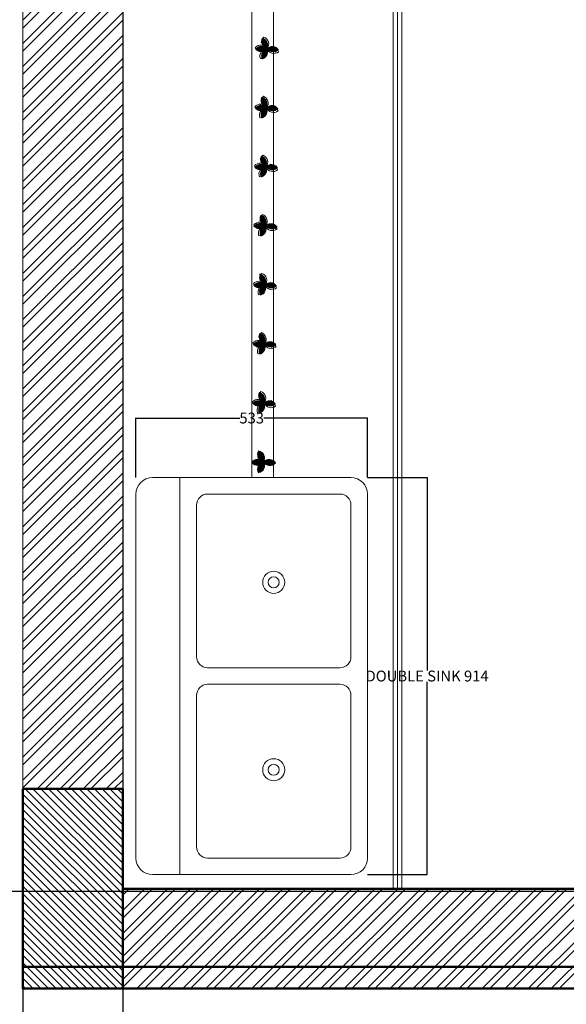
# Model space of a CAD drawing. Units: millimetres. Extents: x 1944 to 29915, y -10550 to 5909.
# Tile 4 of 24: x 6709 to 7967, y -5 to 2263. Entities that reach past the tile are written whole.
import ezdxf
from ezdxf import colors
from ezdxf.entities.mleader import LeaderData, LeaderLine
from ezdxf.math import Vec2, Vec3

# ---------------------------------------------------------------- set-up
doc = ezdxf.new("R2010")
doc.units = ezdxf.units.MM
doc.header["$MEASUREMENT"] = 0
for name, color, linetype, lineweight in [('A-ANNO-DIMS', 2, 'Continuous', 18), ('A-ANNO-TEXT', 7, 'Continuous', 25), ('A-FLOR-FIXT', 9, 'Continuous', 18), ('A-FLOR-PATT', 252, 'Continuous', 13), ('A-WALL', 7, 'Continuous', 50), ('A-WALL-PATT', 8, 'Continuous', 18)]:
    doc.layers.add(name, color=color, linetype=linetype, lineweight=lineweight)
doc.styles.get("Standard").update_dxf_attribs({"font": 'arial.ttf'})
doc.dimstyles.get("Standard").update_dxf_attribs({"dimtxt": 25, "dimasz": 0.18, "dimexe": 0.18, "dimexo": 0.0625, "dimgap": 0.09, "dimtad": 0, "dimtih": 1, "dimtoh": 1, "dimdec": 0, "dimzin": 0, "dimdsep": 46, "dimtxsty": 'Standard', "dimcen": 0.09, "dimadec": 0, "dimazin": 0, "dimtfac": 1, "dimtdec": 0, "dimtofl": 0, "dimtmove": 0, "dimatfit": 3, "dimfxl": 1, "dimtolj": 1, "dimtzin": 0, "dimarcsym": 0})

# ---------------------------------------------------------------- blocks, each defined once
blk = doc.blocks.new('Sink-double - 36 in top')
for p, q in [((-18, -4), (18, -4)), ((-0.75, -18.5), (-0.75, -6.5)), ((0.75, -6.5), (0.75, -18.5))]:
    blk.add_line(p, q)
for points in [[(-16.5, 0), (16.5, 0)], [(-18, -19.5), (-18, -1.5)], [(18, -1.5), (18, -19.5)], [(-15.5, -5.5), (-1.75, -5.5)], [(1.75, -5.5), (15.5, -5.5)], [(-16.5, -18.5), (-16.5, -6.5)], [(16.5, -6.5), (16.5, -18.5)], [(-1.75, -19.5), (-15.5, -19.5)], [(15.5, -19.5), (1.75, -19.5)], [(16.5, -21), (-16.5, -21)]]:
    blk.add_lwpolyline(points)
for centre, radius in [((-8.5, -12.5), 1), ((8.5, -12.5), 1), ((-8.5, -12.5), 0.5), ((8.5, -12.5), 0.5)]:
    blk.add_circle(centre, radius)
for centre, radius, start, end in [((-16.5, -1.5), 1.5, 90, 180), ((16.5, -1.5), 1.5, 0, 90), ((-15.5, -6.5), 1, 90, 180), ((-1.75, -6.5), 1, 0, 90), ((1.75, -6.5), 1, 90, 180), ((15.5, -6.5), 1, 0, 90), ((-15.5, -18.5), 1, 180, 270), ((-1.75, -18.5), 1, 270, 0), ((1.75, -18.5), 1, 180, 270), ((15.5, -18.5), 1, 270, 0), ((-16.5, -19.5), 1.5, 180, 270), ((16.5, -19.5), 1.5, 270, 0)]:
    blk.add_arc(centre, radius, start, end)
blk = doc.blocks.new('ORNAMENT-TILE')
for points in [[(27, 25, 0.520567), (15.6, 50, 0.520567)], [(27.4, 25, -0.520567), (0, 23.1, -0.520567)], [(27, 25, -0.520567), (15.6, 0, -0.520567)], [(27, 25, 0.520567), (54.3, 22.2, 0.520567)]]:
    blk.add_lwpolyline(points, format="xyb", close=True)
blk = doc.blocks.new('*D42')
at = {"layer": 'A-ANNO-DIMS', "color": 0, "lineweight": -2, "transparency": 16777216}
for p, q in [((7509.6, 1208), (7646.9, 1208)), ((7646.7, 1207.8), (7646.7, 763.8)), ((7646.7, 293.7), (7646.7, 737.7)), ((7509.6, 293.6), (7646.9, 293.6))]:
    blk.add_line(p, q, dxfattribs=at)
at = {"layer": 'A-ANNO-DIMS', "color": 0, "transparency": 16777216}
for points in [[(7646.7, 1207.8), (7646.8, 1207.8), (7646.7, 1208)], [(7646.7, 293.7), (7646.8, 293.7), (7646.7, 293.6)]]:
    blk.add_solid(points, dxfattribs=at)
at = {"layer": 'Defpoints', "color": 0, "transparency": 16777216}
for p in [(7509.6, 1208), (7646.7, 1208), (7509.6, 293.6)]:
    blk.add_point(p, dxfattribs=at)
at = {"layer": 'A-ANNO-DIMS', "color": 0, "transparency": 16777216, "insert": (7646.7, 750.8), "char_height": 25, "attachment_point": 5}
blk.add_mtext('\\A1;DOUBLE SINK 914', dxfattribs=at)
blk = doc.blocks.new('*D43')
at = {"layer": 'A-ANNO-DIMS', "color": 0, "lineweight": -2, "transparency": 16777216}
for p, q in [((6976.2, 1208), (6976.2, 1345.3)), ((6976.3, 1345.1), (7215.2, 1345.1)), ((7509.4, 1345.1), (7270.6, 1345.1)), ((7509.6, 1208), (7509.6, 1345.3))]:
    blk.add_line(p, q, dxfattribs=at)
at = {"layer": 'A-ANNO-DIMS', "color": 0, "transparency": 16777216}
for points in [[(6976.3, 1345.2), (6976.3, 1345.1), (6976.2, 1345.1)], [(7509.4, 1345.2), (7509.4, 1345.1), (7509.6, 1345.1)]]:
    blk.add_solid(points, dxfattribs=at)
at = {"layer": 'Defpoints', "color": 0, "transparency": 16777216}
for p in [(6976.2, 1345.1), (6976.2, 1208), (7509.6, 1208)]:
    blk.add_point(p, dxfattribs=at)
at = {"layer": 'A-ANNO-DIMS', "color": 0, "transparency": 16777216, "insert": (7242.9, 1345.1), "char_height": 25, "attachment_point": 5}
blk.add_mtext('\\A1;533', dxfattribs=at)
blk = doc.blocks.new('*D49')
at = {"layer": 'A-ANNO-DIMS', "color": 0, "lineweight": -2, "transparency": 16777216}
for p, q in [((8335.5, 4760.8), (8335.5, -697.2)), ((6945.9, 4530.8), (6945.9, -697.2)), ((6946.1, -697), (7589.8, -697)), ((8335.3, -697), (7691.6, -697))]:
    blk.add_line(p, q, dxfattribs=at)
at = {"layer": 'A-ANNO-DIMS', "color": 0, "transparency": 16777216}
for points in [[(6946.1, -697), (6946.1, -697.1), (6945.9, -697)], [(8335.3, -697), (8335.3, -697.1), (8335.5, -697)]]:
    blk.add_solid(points, dxfattribs=at)
at = {"layer": 'Defpoints', "color": 0, "transparency": 16777216}
for p in [(8335.5, 4760.8), (6945.9, 4530.8), (8335.5, -697)]:
    blk.add_point(p, dxfattribs=at)
at = {"layer": 'A-ANNO-DIMS', "color": 0, "transparency": 16777216, "insert": (7640.7, -697), "char_height": 25, "attachment_point": 5}
blk.add_mtext('\\A1;1389.5', dxfattribs=at)
blk = doc.blocks.new('*D52')
at = {"layer": 'A-ANNO-DIMS', "color": 0, "lineweight": -2, "transparency": 16777216}
for p, q in [((6715.9, 490.8), (6715.9, -697.2)), ((6945.9, 490.8), (6945.9, -697.2)), ((6716.1, -697), (6803.1, -697)), ((6945.8, -697), (6858.8, -697))]:
    blk.add_line(p, q, dxfattribs=at)
at = {"layer": 'A-ANNO-DIMS', "color": 0, "transparency": 16777216}
for points in [[(6716.1, -697), (6716.1, -697.1), (6715.9, -697)], [(6945.8, -697), (6945.8, -697.1), (6945.9, -697)]]:
    blk.add_solid(points, dxfattribs=at)
at = {"layer": 'Defpoints', "color": 0, "transparency": 16777216}
for p in [(6715.9, 490.8), (6945.9, 490.8), (6945.9, -697)]:
    blk.add_point(p, dxfattribs=at)
at = {"layer": 'A-ANNO-DIMS', "color": 0, "transparency": 16777216, "insert": (6830.9, -697), "char_height": 25, "attachment_point": 5}
blk.add_mtext('\\A1;230', dxfattribs=at)
blk = doc.blocks.new('*D53')
at = {"layer": 'A-ANNO-DIMS', "color": 0, "lineweight": -2, "transparency": 16777216}
for p, q in [((6945.94205, 490.774608), (6945.94205, -697.212556)), ((9895.94205, 490.774608), (9895.94205, -697.212556)), ((6946.12205, -697.032556), (8383.35205, -697.032556)), ((9895.76205, -697.032556), (8458.53205, -697.032556))]:
    blk.add_line(p, q, dxfattribs=at)
at = {"layer": 'A-ANNO-DIMS', "color": 0, "transparency": 16777216}
for points in [[(6946.12205, -697.002556), (6946.12205, -697.062556), (6945.94205, -697.032556)], [(9895.76205, -697.002556), (9895.76205, -697.062556), (9895.94205, -697.032556)]]:
    blk.add_solid(points, dxfattribs=at)
at = {"layer": 'Defpoints', "color": 0, "transparency": 16777216}
for p in [(6945.94205, 490.837108), (9895.94205, 490.837108), (9895.94205, -697.032556)]:
    blk.add_point(p, dxfattribs=at)
at = {"layer": 'A-ANNO-DIMS', "color": 0, "transparency": 16777216, "insert": (8420.94205, -697.032556), "char_height": 25, "attachment_point": 5}
blk.add_mtext('\\A1;2950', dxfattribs=at)
blk = doc.blocks.new('*D57')
at = {"layer": 'A-ANNO-DIMS', "color": 0, "lineweight": -2, "transparency": 16777216}
for p, q in [((8995.2, 4760.8), (5803.8, 4760.8)), ((5804, 4760.7), (5804, 2520.7)), ((5804, 255), (5804, 2495)), ((8999.6, 254.8), (5803.8, 254.8))]:
    blk.add_line(p, q, dxfattribs=at)
at = {"layer": 'A-ANNO-DIMS', "color": 0, "transparency": 16777216}
for points in [[(5804, 4760.7), (5804, 4760.7), (5804, 4760.8)], [(5804, 255), (5804, 255), (5804, 254.8)]]:
    blk.add_solid(points, dxfattribs=at)
at = {"layer": 'Defpoints', "color": 0, "transparency": 16777216}
for p in [(8995.2, 4760.8), (5804, 254.8), (8999.6, 254.8)]:
    blk.add_point(p, dxfattribs=at)
at = {"layer": 'A-ANNO-DIMS', "color": 0, "transparency": 16777216, "insert": (5804, 2507.8), "char_height": 25, "attachment_point": 5}
blk.add_mtext('\\A1;4506', dxfattribs=at)

msp = doc.modelspace()

# ---------------------------------------------------------------- hatches: boundary and pattern name
at = {"layer": 'A-FLOR-PATT'}
h = msp.add_hatch(dxfattribs=at)
h.set_pattern_fill('ANSI32', color=256, scale=100)
h.paths.add_polyline_path([(7278.336, 2195.885, -0.00568537), (7278.146, 2196.216, 0.21614784), (7266.8, 2188.29, 0.21566285)], flags=16)
h.paths.add_polyline_path([(7305.459, 2193.46, -0.51336232), (7278.336, 2195.885, -0.51336232), (7266.78, 2171.228, -0.27363046), (7266.8, 2188.29, -0.26802551), (7251.152, 2194.293, -0.30570263), (7268.133, 2202.214, -0.18072738), (7278.345, 2196.442, -0.51487633)])
h.paths.add_polyline_path([(7278.336, 2195.885, -0.21566285), (7266.8, 2188.29, 0.27363046), (7266.78, 2171.228, 0.51336232)], flags=16)
h = msp.add_hatch(dxfattribs=at)
h.set_pattern_fill('ANSI32', color=256, scale=100)
h.paths.add_polyline_path([(7278.146, 2196.216, -0.17977754), (7268.133, 2202.214, 0.30570263), (7251.152, 2194.293, 0.26802551), (7266.8, 2188.29, -0.21614784)])
h.paths.add_polyline_path([(7278.336, 2195.885, -0.00568537), (7278.146, 2196.216, 0.21614784), (7266.8, 2188.29, 0.21566285)], flags=16)
h.paths.add_polyline_path([(7278.336, 2195.885, -0.21566285), (7266.8, 2188.29, 0.27363046), (7266.78, 2171.228, 0.51336232)], flags=16)
h = msp.add_hatch(color=256, dxfattribs=at)
h.dxf.hatch_style = 1
h.paths.add_polyline_path([(7268.133, 2202.214, 0.30570263), (7251.152, 2194.293, 0.26802551), (7266.8, 2188.29, -0.21614784), (7278.146, 2196.216, -0.17977754)])
h = msp.add_hatch(dxfattribs=at)
h.set_pattern_fill('ANSI32', color=256, scale=100)
h.paths.add_polyline_path([(7266.78, 2221.204, 0.31162563), (7268.133, 2202.214, -0.17976414), (7278.304, 2196.49, 0.51458497)])
h = msp.add_hatch(color=256, dxfattribs=at)
h.dxf.hatch_style = 1
h.paths.add_polyline_path([(7266.78, 2221.204, 0.31162563), (7268.133, 2202.214, -0.17976414), (7278.304, 2196.49, 0.51458497)])
h = msp.add_hatch(color=256, dxfattribs=at)
h.dxf.hatch_style = 1
h.paths.add_polyline_path([(7268.133, 2202.214, -0.17976414), (7278.304, 2196.49, 0.51458497), (7266.78, 2221.204, 0.31162563)])
h = msp.add_hatch(color=256, dxfattribs=at)
h.dxf.hatch_style = 1
h.paths.add_polyline_path([(7268.133, 2202.214, 0.17977754), (7278.146, 2196.216, 0.00471819), (7278.304, 2196.49, 0.17976414)])
h = msp.add_hatch(color=256, dxfattribs=at)
h.dxf.hatch_style = 1
h.paths.add_polyline_path([(7278.345, 2196.442, -0.00448785), (7278.536, 2196.21, -0.00568537), (7278.336, 2195.885, 0.51336232), (7305.459, 2193.46, 0.51487633)])
h = msp.add_hatch(color=256, dxfattribs=at)
h.dxf.hatch_style = 1
h.paths.add_polyline_path([(7266.8, 2188.29, 0.27363046), (7266.78, 2171.228, 0.51336232), (7278.336, 2195.885, -0.21566285)])
h = msp.add_hatch(color=256, dxfattribs=at)
h.dxf.hatch_style = 1
h.paths.add_polyline_path([(7278.336, 2195.885, -0.00568537), (7278.146, 2196.216, 0.21614784), (7266.8, 2188.29, 0.21566285)])
h = msp.add_hatch(dxfattribs=at)
h.set_pattern_fill('ANSI32', color=256, scale=100)
h.paths.add_polyline_path([(7277.206, 2059.88, -0.00568537), (7277.016, 2060.21, 0.21614784), (7265.67, 2052.285, 0.21566285)], flags=16)
h.paths.add_polyline_path([(7304.329, 2057.455, -0.51336232), (7277.206, 2059.88, -0.51336232), (7265.651, 2035.222, -0.27363046), (7265.67, 2052.285, -0.26802551), (7250.022, 2058.288, -0.30570263), (7267.004, 2066.209, -0.18072738), (7277.215, 2060.436, -0.51487633)])
h.paths.add_polyline_path([(7277.206, 2059.88, -0.21566285), (7265.67, 2052.285, 0.27363046), (7265.651, 2035.222, 0.51336232)], flags=16)
h = msp.add_hatch(dxfattribs=at)
h.set_pattern_fill('ANSI32', color=256, scale=100)
h.paths.add_polyline_path([(7277.016, 2060.21, -0.17977754), (7267.004, 2066.209, 0.30570263), (7250.022, 2058.288, 0.26802551), (7265.67, 2052.285, -0.21614784)])
h.paths.add_polyline_path([(7277.206, 2059.88, -0.00568537), (7277.016, 2060.21, 0.21614784), (7265.67, 2052.285, 0.21566285)], flags=16)
h.paths.add_polyline_path([(7277.206, 2059.88, -0.21566285), (7265.67, 2052.285, 0.27363046), (7265.651, 2035.222, 0.51336232)], flags=16)
h = msp.add_hatch(color=256, dxfattribs=at)
h.dxf.hatch_style = 1
h.paths.add_polyline_path([(7267.004, 2066.209, 0.30570263), (7250.022, 2058.288, 0.26802551), (7265.67, 2052.285, -0.21614784), (7277.016, 2060.21, -0.17977754)])
h = msp.add_hatch(dxfattribs=at)
h.set_pattern_fill('ANSI32', color=256, scale=100)
h.paths.add_polyline_path([(7265.651, 2085.198, 0.31162563), (7267.004, 2066.209, -0.17976414), (7277.175, 2060.484, 0.51458497)])
h = msp.add_hatch(color=256, dxfattribs=at)
h.dxf.hatch_style = 1
h.paths.add_polyline_path([(7265.651, 2085.198, 0.31162563), (7267.004, 2066.209, -0.17976414), (7277.175, 2060.484, 0.51458497)])
h = msp.add_hatch(color=256, dxfattribs=at)
h.dxf.hatch_style = 1
h.paths.add_polyline_path([(7265.651, 2085.198, 0.31162563), (7267.004, 2066.209, -0.17976414), (7277.175, 2060.484, 0.51458497)])
h = msp.add_hatch(color=256, dxfattribs=at)
h.dxf.hatch_style = 1
h.paths.add_polyline_path([(7267.004, 2066.209, 0.17977754), (7277.016, 2060.21, 0.00471819), (7277.175, 2060.484, 0.17976414)])
h = msp.add_hatch(color=256, dxfattribs=at)
h.dxf.hatch_style = 1
h.paths.add_polyline_path([(7277.215, 2060.436, -0.00448785), (7277.406, 2060.204, -0.00568537), (7277.206, 2059.88, 0.51336232), (7304.329, 2057.455, 0.51487633)])
h = msp.add_hatch(color=256, dxfattribs=at)
h.dxf.hatch_style = 1
h.paths.add_polyline_path([(7265.67, 2052.285, 0.27363046), (7265.651, 2035.222, 0.51336232), (7277.206, 2059.88, -0.21566285)])
h = msp.add_hatch(color=256, dxfattribs=at)
h.dxf.hatch_style = 1
h.paths.add_polyline_path([(7277.206, 2059.88, -0.00568537), (7277.016, 2060.21, 0.21614784), (7265.67, 2052.285, 0.21566285)])
h = msp.add_hatch(dxfattribs=at)
h.set_pattern_fill('ANSI32', color=256, scale=100)
h.paths.add_polyline_path([(7276.077, 1923.875, -0.00568537), (7275.887, 1924.205, 0.21614784), (7264.54, 1916.279, 0.21566285)], flags=16)
h.paths.add_polyline_path([(7303.199, 1921.449, -0.51336232), (7276.077, 1923.875, -0.51336232), (7264.521, 1899.217, -0.27363046), (7264.54, 1916.279, -0.26802551), (7248.892, 1922.282, -0.30570263), (7265.874, 1930.203, -0.18072738), (7276.085, 1924.431, -0.51487633)])
h.paths.add_polyline_path([(7276.077, 1923.875, -0.21566285), (7264.54, 1916.279, 0.27363046), (7264.521, 1899.217, 0.51336232)], flags=16)
h = msp.add_hatch(dxfattribs=at)
h.set_pattern_fill('ANSI32', color=256, scale=100)
h.paths.add_polyline_path([(7275.887, 1924.205, -0.17977754), (7265.874, 1930.203, 0.30570263), (7248.892, 1922.282, 0.26802551), (7264.54, 1916.279, -0.21614784)])
h.paths.add_polyline_path([(7276.077, 1923.875, -0.00568537), (7275.887, 1924.205, 0.21614784), (7264.54, 1916.279, 0.21566285)], flags=16)
h.paths.add_polyline_path([(7276.077, 1923.875, -0.21566285), (7264.54, 1916.279, 0.27363046), (7264.521, 1899.217, 0.51336232)], flags=16)
h = msp.add_hatch(color=256, dxfattribs=at)
h.dxf.hatch_style = 1
h.paths.add_polyline_path([(7265.874, 1930.203, 0.30570263), (7248.892, 1922.282, 0.26802551), (7264.54, 1916.279, -0.21614784), (7275.887, 1924.205, -0.17977754)])
h = msp.add_hatch(dxfattribs=at)
h.set_pattern_fill('ANSI32', color=256, scale=100)
h.paths.add_polyline_path([(7264.521, 1949.193, 0.31162563), (7265.874, 1930.203, -0.17976414), (7276.045, 1924.479, 0.51458497)])
h = msp.add_hatch(color=256, dxfattribs=at)
h.dxf.hatch_style = 1
h.paths.add_polyline_path([(7264.521, 1949.193, 0.31162563), (7265.874, 1930.203, -0.17976414), (7276.045, 1924.479, 0.51458497)])
h = msp.add_hatch(color=256, dxfattribs=at)
h.dxf.hatch_style = 1
h.paths.add_polyline_path([(7264.521, 1949.193, 0.31162563), (7265.874, 1930.203, -0.17976414), (7276.045, 1924.479, 0.51458497)])
h = msp.add_hatch(color=256, dxfattribs=at)
h.dxf.hatch_style = 1
h.paths.add_polyline_path([(7265.874, 1930.203, 0.17977754), (7275.887, 1924.205, 0.00471819), (7276.045, 1924.479, 0.17976414)])
h = msp.add_hatch(color=256, dxfattribs=at)
h.dxf.hatch_style = 1
h.paths.add_polyline_path([(7276.085, 1924.431, -0.00448785), (7276.276, 1924.199, -0.00568537), (7276.077, 1923.875, 0.51336232), (7303.199, 1921.449, 0.51487633)])
h = msp.add_hatch(color=256, dxfattribs=at)
h.dxf.hatch_style = 1
h.paths.add_polyline_path([(7264.54, 1916.279, 0.27363046), (7264.521, 1899.217, 0.51336232), (7276.077, 1923.875, -0.21566285)])
h = msp.add_hatch(color=256, dxfattribs=at)
h.dxf.hatch_style = 1
h.paths.add_polyline_path([(7276.077, 1923.875, -0.00568537), (7275.887, 1924.205, 0.21614784), (7264.54, 1916.279, 0.21566285)])
h = msp.add_hatch(dxfattribs=at)
h.set_pattern_fill('ANSI32', color=256, scale=100)
h.paths.add_polyline_path([(7274.947, 1787.869, -0.00568537), (7274.757, 1788.2, 0.21614784), (7263.41, 1780.274, 0.21566285)], flags=16)
h.paths.add_polyline_path([(7302.069, 1785.444, -0.51336232), (7274.947, 1787.869, -0.51336232), (7263.391, 1763.212, -0.27363046), (7263.41, 1780.274, -0.26802551), (7247.762, 1786.277, -0.30570263), (7264.744, 1794.198, -0.18072738), (7274.955, 1788.426, -0.51487633)])
h.paths.add_polyline_path([(7274.947, 1787.869, -0.21566285), (7263.41, 1780.274, 0.27363046), (7263.391, 1763.212, 0.51336232)], flags=16)
h = msp.add_hatch(dxfattribs=at)
h.set_pattern_fill('ANSI32', color=256, scale=100)
h.paths.add_polyline_path([(7274.757, 1788.2, -0.17977754), (7264.744, 1794.198, 0.30570263), (7247.762, 1786.277, 0.26802551), (7263.41, 1780.274, -0.21614784)])
h.paths.add_polyline_path([(7274.947, 1787.869, -0.00568537), (7274.757, 1788.2, 0.21614784), (7263.41, 1780.274, 0.21566285)], flags=16)
h.paths.add_polyline_path([(7274.947, 1787.869, -0.21566285), (7263.41, 1780.274, 0.27363046), (7263.391, 1763.212, 0.51336232)], flags=16)
h = msp.add_hatch(color=256, dxfattribs=at)
h.dxf.hatch_style = 1
h.paths.add_polyline_path([(7264.744, 1794.198, 0.30570263), (7247.762, 1786.277, 0.26802551), (7263.41, 1780.274, -0.21614784), (7274.757, 1788.2, -0.17977754)])
h = msp.add_hatch(dxfattribs=at)
h.set_pattern_fill('ANSI32', color=256, scale=100)
h.paths.add_polyline_path([(7263.391, 1813.187, 0.31162563), (7264.744, 1794.198, -0.17976414), (7274.915, 1788.473, 0.51458497)])
h = msp.add_hatch(color=256, dxfattribs=at)
h.dxf.hatch_style = 1
h.paths.add_polyline_path([(7263.391, 1813.187, 0.31162563), (7264.744, 1794.198, -0.17976414), (7274.915, 1788.473, 0.51458497)])
h = msp.add_hatch(color=256, dxfattribs=at)
h.dxf.hatch_style = 1
h.paths.add_polyline_path([(7274.915, 1788.473, 0.51458497), (7263.391, 1813.187, 0.31162563), (7264.744, 1794.198, -0.17976414)])
h = msp.add_hatch(color=256, dxfattribs=at)
h.dxf.hatch_style = 1
h.paths.add_polyline_path([(7264.744, 1794.198, 0.17977754), (7274.757, 1788.2, 0.00471819), (7274.915, 1788.473, 0.17976414)])
h = msp.add_hatch(color=256, dxfattribs=at)
h.dxf.hatch_style = 1
h.paths.add_polyline_path([(7274.955, 1788.426, -0.00448785), (7275.147, 1788.194, -0.00568537), (7274.947, 1787.869, 0.51336232), (7302.069, 1785.444, 0.51487633)])
h = msp.add_hatch(color=256, dxfattribs=at)
h.dxf.hatch_style = 1
h.paths.add_polyline_path([(7263.41, 1780.274, 0.27363046), (7263.391, 1763.212, 0.51336232), (7274.947, 1787.869, -0.21566285)])
h = msp.add_hatch(color=256, dxfattribs=at)
h.dxf.hatch_style = 1
h.paths.add_polyline_path([(7274.947, 1787.869, -0.00568537), (7274.757, 1788.2, 0.21614784), (7263.41, 1780.274, 0.21566285)])
h = msp.add_hatch(dxfattribs=at)
h.set_pattern_fill('ANSI32', color=256, scale=100)
h.paths.add_polyline_path([(7273.817, 1651.864, -0.00568537), (7273.627, 1652.194, 0.21614784), (7262.281, 1644.268, 0.21566285)], flags=16)
h.paths.add_polyline_path([(7300.94, 1649.438, -0.51336232), (7273.817, 1651.864, -0.51336232), (7262.261, 1627.206, -0.27363046), (7262.281, 1644.268, -0.26802551), (7246.633, 1650.272, -0.30570263), (7263.614, 1658.193, -0.18072738), (7273.825, 1652.42, -0.51487633)])
h.paths.add_polyline_path([(7273.817, 1651.864, -0.21566285), (7262.281, 1644.268, 0.27363046), (7262.261, 1627.206, 0.51336232)], flags=16)
h = msp.add_hatch(dxfattribs=at)
h.set_pattern_fill('ANSI32', color=256, scale=100)
h.paths.add_polyline_path([(7273.627, 1652.194, -0.17977754), (7263.614, 1658.193, 0.30570263), (7246.633, 1650.272, 0.26802551), (7262.281, 1644.268, -0.21614784)])
h.paths.add_polyline_path([(7273.817, 1651.864, -0.00568537), (7273.627, 1652.194, 0.21614784), (7262.281, 1644.268, 0.21566285)], flags=16)
h.paths.add_polyline_path([(7273.817, 1651.864, -0.21566285), (7262.281, 1644.268, 0.27363046), (7262.261, 1627.206, 0.51336232)], flags=16)
h = msp.add_hatch(color=256, dxfattribs=at)
h.dxf.hatch_style = 1
h.paths.add_polyline_path([(7263.614, 1658.193, 0.30570263), (7246.633, 1650.272, 0.26802551), (7262.281, 1644.268, -0.21614784), (7273.627, 1652.194, -0.17977754)])
h = msp.add_hatch(dxfattribs=at)
h.set_pattern_fill('ANSI32', color=256, scale=100)
h.paths.add_polyline_path([(7262.261, 1677.182, 0.31162563), (7263.614, 1658.193, -0.17976414), (7273.785, 1652.468, 0.51458497)])
h = msp.add_hatch(color=256, dxfattribs=at)
h.dxf.hatch_style = 1
h.paths.add_polyline_path([(7262.261, 1677.182, 0.31162563), (7263.614, 1658.193, -0.17976414), (7273.785, 1652.468, 0.51458497)])
h = msp.add_hatch(color=256, dxfattribs=at)
h.dxf.hatch_style = 1
h.paths.add_polyline_path([(7262.261, 1677.182, 0.31162563), (7263.614, 1658.193, -0.17976414), (7273.785, 1652.468, 0.51458497)])
h = msp.add_hatch(color=256, dxfattribs=at)
h.dxf.hatch_style = 1
h.paths.add_polyline_path([(7263.614, 1658.193, 0.17977754), (7273.627, 1652.194, 0.00471819), (7273.785, 1652.468, 0.17976414)])
h = msp.add_hatch(color=256, dxfattribs=at)
h.dxf.hatch_style = 1
h.paths.add_polyline_path([(7273.825, 1652.42, -0.00448785), (7274.017, 1652.188, -0.00568537), (7273.817, 1651.864, 0.51336232), (7300.94, 1649.438, 0.51487633)])
h = msp.add_hatch(color=256, dxfattribs=at)
h.dxf.hatch_style = 1
h.paths.add_polyline_path([(7262.281, 1644.268, 0.27363046), (7262.261, 1627.206, 0.51336232), (7273.817, 1651.864, -0.21566285)])
h = msp.add_hatch(color=256, dxfattribs=at)
h.dxf.hatch_style = 1
h.paths.add_polyline_path([(7273.817, 1651.864, -0.00568537), (7273.627, 1652.194, 0.21614784), (7262.281, 1644.268, 0.21566285)])
h = msp.add_hatch(dxfattribs=at)
h.set_pattern_fill('ANSI32', color=256, scale=100)
h.paths.add_polyline_path([(7272.687, 1515.858, -0.00568537), (7272.497, 1516.189, 0.21614784), (7261.151, 1508.263, 0.21566285)], flags=16)
h.paths.add_polyline_path([(7299.81, 1513.433, -0.51336232), (7272.687, 1515.858, -0.51336232), (7261.131, 1491.201, -0.27363046), (7261.151, 1508.263, -0.26802551), (7245.503, 1514.266, -0.30570263), (7262.484, 1522.187, -0.18072738), (7272.696, 1516.415, -0.51487633)])
h.paths.add_polyline_path([(7272.687, 1515.858, -0.21566285), (7261.151, 1508.263, 0.27363046), (7261.131, 1491.201, 0.51336232)], flags=16)
h = msp.add_hatch(dxfattribs=at)
h.set_pattern_fill('ANSI32', color=256, scale=100)
h.paths.add_polyline_path([(7272.497, 1516.189, -0.17977754), (7262.484, 1522.187, 0.30570263), (7245.503, 1514.266, 0.26802551), (7261.151, 1508.263, -0.21614784)])
h.paths.add_polyline_path([(7272.687, 1515.858, -0.00568537), (7272.497, 1516.189, 0.21614784), (7261.151, 1508.263, 0.21566285)], flags=16)
h.paths.add_polyline_path([(7272.687, 1515.858, -0.21566285), (7261.151, 1508.263, 0.27363046), (7261.131, 1491.201, 0.51336232)], flags=16)
h = msp.add_hatch(color=256, dxfattribs=at)
h.dxf.hatch_style = 1
h.paths.add_polyline_path([(7262.484, 1522.187, 0.30570263), (7245.503, 1514.266, 0.26802551), (7261.151, 1508.263, -0.21614784), (7272.497, 1516.189, -0.17977754)])
h = msp.add_hatch(dxfattribs=at)
h.set_pattern_fill('ANSI32', color=256, scale=100)
h.paths.add_polyline_path([(7261.131, 1541.177, 0.31162563), (7262.484, 1522.187, -0.17976414), (7272.655, 1516.463, 0.51458497)])
h = msp.add_hatch(color=256, dxfattribs=at)
h.dxf.hatch_style = 1
h.paths.add_polyline_path([(7261.131, 1541.177, 0.31162563), (7262.484, 1522.187, -0.17976414), (7272.655, 1516.463, 0.51458497)])
h = msp.add_hatch(color=256, dxfattribs=at)
h.dxf.hatch_style = 1
h.paths.add_polyline_path([(7261.131, 1541.177, 0.31162563), (7262.484, 1522.187, -0.17976414), (7272.655, 1516.463, 0.51458497)])
h = msp.add_hatch(color=256, dxfattribs=at)
h.dxf.hatch_style = 1
h.paths.add_polyline_path([(7262.484, 1522.187, 0.17977754), (7272.497, 1516.189, 0.00471819), (7272.655, 1516.463, 0.17976414)])
h = msp.add_hatch(color=256, dxfattribs=at)
h.dxf.hatch_style = 1
h.paths.add_polyline_path([(7272.696, 1516.415, -0.00448785), (7272.887, 1516.183, -0.00568537), (7272.687, 1515.858, 0.51336232), (7299.81, 1513.433, 0.51487633)])
h = msp.add_hatch(color=256, dxfattribs=at)
h.dxf.hatch_style = 1
h.paths.add_polyline_path([(7261.151, 1508.263, 0.27363046), (7261.131, 1491.201, 0.51336232), (7272.687, 1515.858, -0.21566285)])
h = msp.add_hatch(color=256, dxfattribs=at)
h.dxf.hatch_style = 1
h.paths.add_polyline_path([(7272.687, 1515.858, -0.00568537), (7272.497, 1516.189, 0.21614784), (7261.151, 1508.263, 0.21566285)])
h = msp.add_hatch(dxfattribs=at)
h.set_pattern_fill('ANSI32', color=256, scale=100)
h.paths.add_polyline_path([(7271.557, 1379.853, -0.00568537), (7271.367, 1380.183, 0.21614784), (7260.021, 1372.258, 0.21566285)], flags=16)
h.paths.add_polyline_path([(7298.68, 1377.428, -0.51336232), (7271.557, 1379.853, -0.51336232), (7260.002, 1355.195, -0.27363046), (7260.021, 1372.258, -0.26802551), (7244.373, 1378.261, -0.30570263), (7261.355, 1386.182, -0.18072738), (7271.566, 1380.409, -0.51487633)])
h.paths.add_polyline_path([(7271.557, 1379.853, -0.21566285), (7260.021, 1372.258, 0.27363046), (7260.002, 1355.195, 0.51336232)], flags=16)
h = msp.add_hatch(dxfattribs=at)
h.set_pattern_fill('ANSI32', color=256, scale=100)
h.paths.add_polyline_path([(7271.367, 1380.183, -0.17977754), (7261.355, 1386.182, 0.30570263), (7244.373, 1378.261, 0.26802551), (7260.021, 1372.258, -0.21614784)])
h.paths.add_polyline_path([(7271.557, 1379.853, -0.00568537), (7271.367, 1380.183, 0.21614784), (7260.021, 1372.258, 0.21566285)], flags=16)
h.paths.add_polyline_path([(7271.557, 1379.853, -0.21566285), (7260.021, 1372.258, 0.27363046), (7260.002, 1355.195, 0.51336232)], flags=16)
h = msp.add_hatch(color=256, dxfattribs=at)
h.dxf.hatch_style = 1
h.paths.add_polyline_path([(7261.355, 1386.182, 0.30570263), (7244.373, 1378.261, 0.26802551), (7260.021, 1372.258, -0.21614784), (7271.367, 1380.183, -0.17977754)])
h = msp.add_hatch(dxfattribs=at)
h.set_pattern_fill('ANSI32', color=256, scale=100)
h.paths.add_polyline_path([(7260.002, 1405.171, 0.31162563), (7261.355, 1386.182, -0.17976414), (7271.526, 1380.457, 0.51458497)])
h = msp.add_hatch(color=256, dxfattribs=at)
h.dxf.hatch_style = 1
h.paths.add_polyline_path([(7260.002, 1405.171, 0.31162563), (7261.355, 1386.182, -0.17976414), (7271.526, 1380.457, 0.51458497)])
h = msp.add_hatch(color=256, dxfattribs=at)
h.dxf.hatch_style = 1
h.paths.add_polyline_path([(7260.002, 1405.171, 0.31162563), (7261.355, 1386.182, -0.17976414), (7271.526, 1380.457, 0.51458497)])
h = msp.add_hatch(color=256, dxfattribs=at)
h.dxf.hatch_style = 1
h.paths.add_polyline_path([(7261.355, 1386.182, 0.17977754), (7271.367, 1380.183, 0.00471819), (7271.526, 1380.457, 0.17976414)])
h = msp.add_hatch(color=256, dxfattribs=at)
h.dxf.hatch_style = 1
h.paths.add_polyline_path([(7271.566, 1380.409, -0.00448785), (7271.757, 1380.177, -0.00568537), (7271.557, 1379.853, 0.51336232), (7298.68, 1377.428, 0.51487633)])
h = msp.add_hatch(color=256, dxfattribs=at)
h.dxf.hatch_style = 1
h.paths.add_polyline_path([(7260.021, 1372.258, 0.27363046), (7260.002, 1355.195, 0.51336232), (7271.557, 1379.853, -0.21566285)])
h = msp.add_hatch(color=256, dxfattribs=at)
h.dxf.hatch_style = 1
h.paths.add_polyline_path([(7271.557, 1379.853, -0.00568537), (7271.367, 1380.183, 0.21614784), (7260.021, 1372.258, 0.21566285)])
h = msp.add_hatch(dxfattribs=at)
h.set_pattern_fill('ANSI32', color=256, scale=100)
h.paths.add_polyline_path([(7270.428, 1243.848, -0.00568537), (7270.238, 1244.178, 0.21614784), (7258.891, 1236.252, 0.21566285)], flags=16)
h.paths.add_polyline_path([(7297.55, 1241.422, -0.51336232), (7270.428, 1243.848, -0.51336232), (7258.872, 1219.19, -0.27363046), (7258.891, 1236.252, -0.26802551), (7243.243, 1242.255, -0.30570263), (7260.225, 1250.176, -0.18072738), (7270.436, 1244.404, -0.51487633)])
h.paths.add_polyline_path([(7270.428, 1243.848, -0.21566285), (7258.891, 1236.252, 0.27363046), (7258.872, 1219.19, 0.51336232)], flags=16)
h = msp.add_hatch(dxfattribs=at)
h.set_pattern_fill('ANSI32', color=256, scale=100)
h.paths.add_polyline_path([(7270.238, 1244.178, -0.17977754), (7260.225, 1250.176, 0.30570263), (7243.243, 1242.255, 0.26802551), (7258.891, 1236.252, -0.21614784)])
h.paths.add_polyline_path([(7270.428, 1243.848, -0.00568537), (7270.238, 1244.178, 0.21614784), (7258.891, 1236.252, 0.21566285)], flags=16)
h.paths.add_polyline_path([(7270.428, 1243.848, -0.21566285), (7258.891, 1236.252, 0.27363046), (7258.872, 1219.19, 0.51336232)], flags=16)
h = msp.add_hatch(color=256, dxfattribs=at)
h.dxf.hatch_style = 1
h.paths.add_polyline_path([(7260.225, 1250.176, 0.30570263), (7243.243, 1242.255, 0.26802551), (7258.891, 1236.252, -0.21614784), (7270.238, 1244.178, -0.17977754)])
h = msp.add_hatch(dxfattribs=at)
h.set_pattern_fill('ANSI32', color=256, scale=100)
h.paths.add_polyline_path([(7258.872, 1269.166, 0.31162563), (7260.225, 1250.176, -0.17976414), (7270.396, 1244.452, 0.51458497)])
h = msp.add_hatch(color=256, dxfattribs=at)
h.dxf.hatch_style = 1
h.paths.add_polyline_path([(7258.872, 1269.166, 0.31162563), (7260.225, 1250.176, -0.17976414), (7270.396, 1244.452, 0.51458497)])
h = msp.add_hatch(color=256, dxfattribs=at)
h.dxf.hatch_style = 1
h.paths.add_polyline_path([(7258.872, 1269.166, 0.31162563), (7260.225, 1250.176, -0.17976414), (7270.396, 1244.452, 0.51458497)])
h = msp.add_hatch(color=256, dxfattribs=at)
h.dxf.hatch_style = 1
h.paths.add_polyline_path([(7260.225, 1250.176, 0.17977754), (7270.238, 1244.178, 0.00471819), (7270.396, 1244.452, 0.17976414)])
h = msp.add_hatch(color=256, dxfattribs=at)
h.dxf.hatch_style = 1
h.paths.add_polyline_path([(7270.436, 1244.404, -0.00448785), (7270.627, 1244.172, -0.00568537), (7270.428, 1243.848, 0.51336232), (7297.55, 1241.422, 0.51487633)])
h = msp.add_hatch(color=256, dxfattribs=at)
h.dxf.hatch_style = 1
h.paths.add_polyline_path([(7258.891, 1236.252, 0.27363046), (7258.872, 1219.19, 0.51336232), (7270.428, 1243.848, -0.21566285)])
h = msp.add_hatch(color=256, dxfattribs=at)
h.dxf.hatch_style = 1
h.paths.add_polyline_path([(7270.428, 1243.848, -0.00568537), (7270.238, 1244.178, 0.21614784), (7258.891, 1236.252, 0.21566285)])
at = {"layer": 'A-WALL-PATT'}
h = msp.add_hatch(dxfattribs=at)
h.set_pattern_fill('ANSI32', color=256, scale=100)
h.paths.add_polyline_path([(6945.942, 4530.837), (6715.942, 4530.837), (6715.942, 490.837), (6945.942, 490.837)])
h = msp.add_hatch(dxfattribs=at)
h.set_pattern_fill('ANSI31', color=256, scale=100, angle=90)
h.paths.add_polyline_path([(6715.942, 30.837), (6945.942, 30.837), (6945.942, 490.837), (6715.942, 490.837)])
h = msp.add_hatch(dxfattribs=at)
h.set_pattern_fill('ANSI32', color=256, scale=100)
h.paths.add_polyline_path([(6945.942, 260.837), (6945.942, 30.837), (8995.217, 30.837), (8995.217, 165.837, -0.0264443), (9000.245, 260.837)])

# ---------------------------------------------------------------- linework, layer by layer
at = {"layer": 'A-FLOR-FIXT'}
for p, q in [((7242.862, 1207.97), (7242.862, 3860.837)), ((7292.862, 1207.97), (7292.862, 3860.837)), ((7568.787, 3860.837), (7568.787, 260.837)), ((7578.787, 3860.837), (7578.787, 260.837)), ((7578.787, 3860.837), (7578.787, 260.837)), ((7588.787, 3860.837), (7588.787, 260.837))]:
    msp.add_line(p, q, dxfattribs=at)
for points in [[(8995.217, 30.837), (6715.942, 30.837), (6715.942, 4990.837), (8315.477, 4990.837)], [(9000.245, 260.837), (6945.942, 260.837), (6945.942, 4760.837), (8315.477, 4760.837)]]:
    msp.add_lwpolyline(points, dxfattribs=at)
at = {"layer": 'A-WALL'}
for p, q in [((6945.942, 260.837), (9000.245, 260.837)), ((6945.942, 260.837), (7845.942, 260.837)), ((10125.942, 81.017), (6715.942, 81.017)), ((10125.942, 30.837), (6715.942, 30.837))]:
    msp.add_line(p, q, dxfattribs=at)
msp.add_lwpolyline([(6715.942, 490.837), (6945.942, 490.837), (6945.942, 30.837), (6715.942, 30.837)], close=True, dxfattribs=at)

# ---------------------------------------------------------------- block references
at = {"layer": 'A-FLOR-FIXT', "xscale": 25.4, "yscale": 25.4, "zscale": 25.4, "rotation": 90}
msp.add_blockref('Sink-double - 36 in top', (6976.162, 750.77), dxfattribs=at)
at = {"layer": 'A-FLOR-PATT'}
for p, rotation in [((7247.597, 2175.381), 350.9047073759607), ((7246.467, 2039.375), 350.9047073759602), ((7245.338, 1903.37), 350.904707375964), ((7244.208, 1767.364), 350.9047073759601), ((7243.078, 1631.359), 350.9047073759621), ((7241.948, 1495.354), 350.9047073759601), ((7240.818, 1359.348), 350.904707375963)]:
    msp.add_blockref('ORNAMENT-TILE', p, dxfattribs=dict(at, rotation=rotation))
msp.add_blockref('ORNAMENT-TILE', (7243.243, 1219.19), dxfattribs=at)

# ---------------------------------------------------------------- dimensions: what is measured, and where the dimension line sits
at = {"layer": 'A-ANNO-DIMS'}
for base, p1, p2, angle, override, picture, middle in [((5803.984, 254.791), (8995.217, 4760.837), (8999.621, 254.791), 90, {"dimdec": 0, "dimlfac": 1, "dimrnd": 0, "dimzin": 0, "dimdsep": 46, "dimlunit": 2}, '*D57', (5803.984, 2507.814)), ((6976.162, 1345.13), (7509.562, 1207.97), (6976.162, 1207.97), 180, {"dimdec": 0, "dimrnd": 0, "dimzin": 0, "dimlunit": 2}, '*D43', (7242.862, 1345.13))]:
    dim = msp.add_linear_dim(base=base, p1=p1, p2=p2, angle=angle, dimstyle='Standard', override=override, dxfattribs=at)
    dim.commit()
    dim.dimension.update_dxf_attribs({"geometry": picture, "text_midpoint": middle})
for base, p1, p2, override, picture, middle in [((8335.477, -697.033), (6945.942, 4530.837), (8335.477, 4760.837), {"dimdec": 1, "dimlfac": 1, "dimrnd": 0, "dimzin": 0, "dimdsep": 46, "dimlunit": 2}, '*D49', (7640.71, -697.033)), ((6945.942, -697.033), (6715.942, 490.837), (6945.942, 490.837), {"dimdec": 0, "dimlfac": 1, "dimrnd": 0, "dimzin": 0, "dimdsep": 46, "dimlunit": 2}, '*D52', (6830.942, -697.033)), ((9895.942, -697.033), (6945.942, 490.837), (9895.942, 490.837), {"dimdec": 0, "dimlfac": 1, "dimrnd": 0, "dimzin": 0, "dimdsep": 46, "dimlunit": 2}, '*D53', (8420.942, -697.033))]:
    dim = msp.add_linear_dim(base=base, p1=p1, p2=p2, dimstyle='Standard', override=override, dxfattribs=at)
    dim.commit()
    dim.dimension.update_dxf_attribs({"geometry": picture, "text_midpoint": middle})
dim = msp.add_linear_dim(base=(7646.722, 1207.97), p1=(7509.562, 293.57), p2=(7509.562, 1207.97), angle=90, text='DOUBLE SINK <>', dimstyle='Standard', override={"dimdec": 0, "dimrnd": 0, "dimzin": 0, "dimlunit": 2}, dxfattribs=at)
dim.commit()
dim.dimension.update_dxf_attribs({"geometry": '*D42', "text_midpoint": (7646.722, 750.77)})

# ---------------------------------------------------------------- leaders
at = {"layer": 'A-ANNO-TEXT'}
ml = msp.add_multileader_mtext('Standard', dxfattribs=at)
ml.set_content('15 AMP POWER POINT \\PFOR MIXER', color=256)
ml.set_leader_properties()
ml.build(insert=Vec2(0, 0))
ml.multileader.update_dxf_attribs({"dogleg_length": 568.936, "arrow_head_size": 100})
ctx = ml.context
ctx.base_point, ctx.char_height, ctx.arrow_head_size, ctx.landing_gap_size, ctx.plane_origin = Vec3(4878.252, -422.117), 100, 100, 0.09, Vec3(6870.097, -798.764)
ctx.text_align_type = 2
notes = []
notes.append((ctx, [(0, (1, 1, 0), (6958.555, -422.117), (-1, 0), 568.936, [(0, [(8384.052, 260.837), (8397.606, -446.246)], 0, [])])]))
ctx.mtext.insert, ctx.mtext.alignment, ctx.mtext.flow_direction = Vec3(6389.529, -371.264), 3, 5
for ctx, leaders in notes:
    for number, flags, end, landing, length, lines in leaders:
        leader = LeaderData()
        leader.index, (leader.has_last_leader_line, leader.has_dogleg_vector, leader.attachment_direction) = number, flags
        leader.last_leader_point, leader.dogleg_vector, leader.dogleg_length = Vec3(end), Vec3(landing), length
        for number, points, colour, breaks in lines:
            line = LeaderLine()
            line.index, line.vertices, line.color, line.breaks = number, Vec3.list(points), colors.encode_raw_color(colour), breaks
            leader.lines.append(line)
        ctx.leaders.append(leader)

doc.saveas('drawing.dxf')
